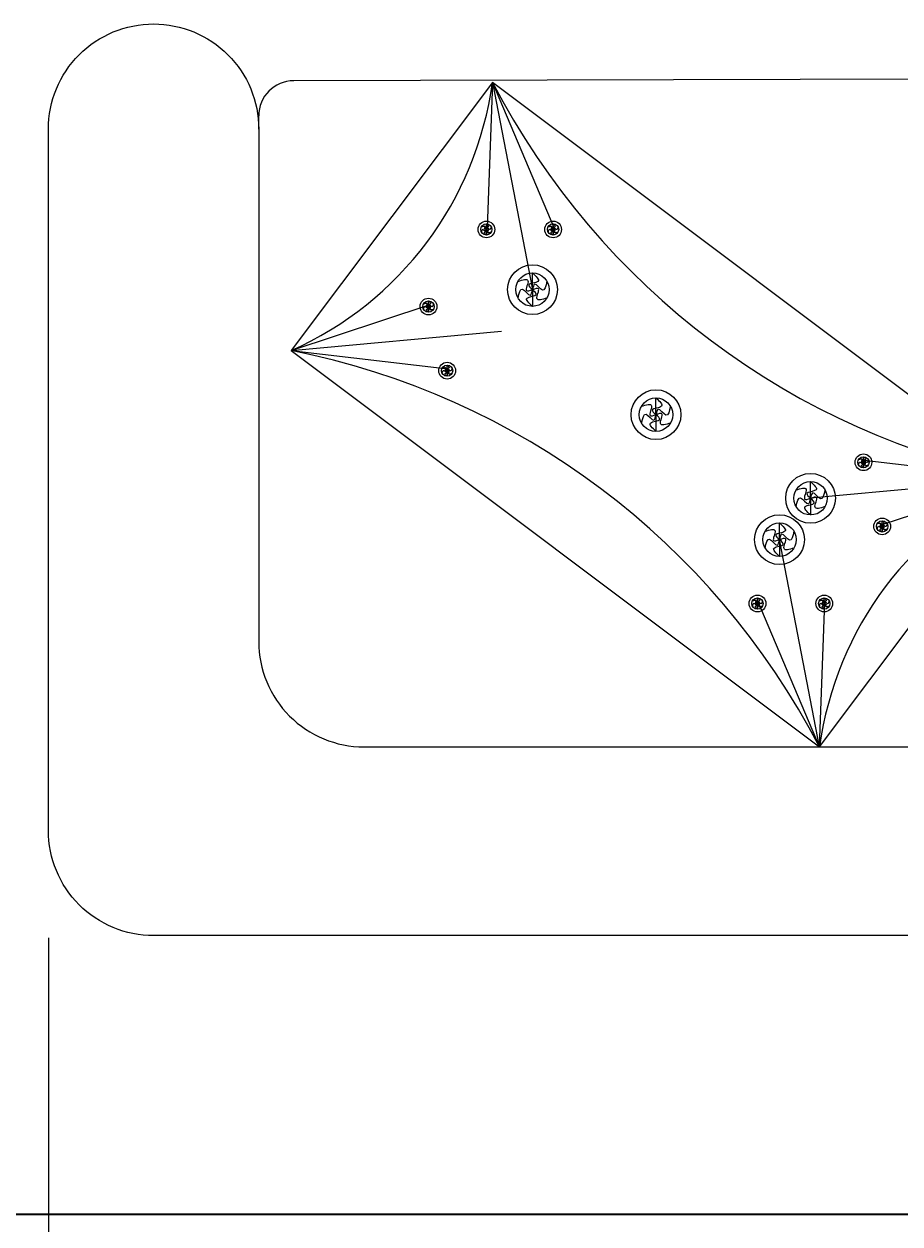
# Model space of a CAD drawing. Units: inches. Extents: x -61 to 1599, y -1316 to 257.
# Tile 163 of 204: x 1123 to 1148, y -939 to -905. Entities that reach past the tile are written whole.
import ezdxf

# ---------------------------------------------------------------- set-up
doc = ezdxf.new("R2010")
doc.units = ezdxf.units.IN
doc.header["$MEASUREMENT"] = 0
for name, color, linetype, lineweight in [('A-ANNO-DIMS', 2, 'Continuous', 18), ('FURNITURE', 83, 'Continuous', 18), ('WALLS', 4, 'Continuous', 35)]:
    doc.layers.add(name, color=color, linetype=linetype, lineweight=lineweight)
doc.layers.add('FUR', color=83, linetype='Continuous')
doc.styles.get("Standard").update_dxf_attribs({"font": 'arial.ttf'})
doc.dimstyles.get("Standard").update_dxf_attribs({"dimtxt": 0.18, "dimasz": 0.18, "dimexe": 0.18, "dimexo": 0.0625, "dimgap": 0.09, "dimtad": 0, "dimtih": 1, "dimtoh": 1, "dimdec": 0, "dimzin": 0, "dimdsep": 46, "dimlunit": 3, "dimtxsty": 'Standard', "dimcen": 0.09, "dimadec": 0, "dimazin": 0, "dimtfac": 1, "dimtdec": 0, "dimtofl": 0, "dimtmove": 0, "dimatfit": 3, "dimfxl": 1, "dimtolj": 1, "dimtzin": 0, "dimarcsym": 0})

# ---------------------------------------------------------------- blocks, each defined once
blk = doc.blocks.new('*U514')
at = {"layer": 'FUR'}
blk.add_open_spline([(0.005, 0.08), (-0.03, 0.048), (-0.098, -0.015), (0.075, -0.018), (0.024, -0.063), (0.005, -0.08)], degree=3, knots=[0, 0, 0, 0, 0.0954578, 0.1898773, 0.2470677, 0.2470677, 0.2470677, 0.2470677], dxfattribs=at)
blk = doc.blocks.new('*U515')
at = {"layer": 'FUR', "transparency": 16777216}
for p, rotation in [((222.173, -79.977), 60), ((222.178, -80.056), 120), ((222.25, -80.092), 180), ((222.312, -79.968), 300), ((222.317, -80.048), 240)]:
    blk.add_blockref('*U514', p, dxfattribs=dict(at, rotation=rotation))
blk.add_blockref('*U514', (222.24, -79.932), dxfattribs=at)
blk = doc.blocks.new('*U516')
at = {"layer": 'FUR'}
blk.add_open_spline([(0.005, 0.08), (-0.03, 0.048), (-0.098, -0.015), (0.075, -0.018), (0.024, -0.063), (0.005, -0.08)], degree=3, knots=[0, 0, 0, 0, 0.0954578, 0.1898773, 0.2470677, 0.2470677, 0.2470677, 0.2470677], dxfattribs=at)
blk = doc.blocks.new('*U517')
at = {"layer": 'FUR', "transparency": 16777216}
for p, rotation in [((222.173, -79.977), 60), ((222.178, -80.056), 120), ((222.25, -80.092), 180), ((222.312, -79.968), 300), ((222.317, -80.048), 240)]:
    blk.add_blockref('*U516', p, dxfattribs=dict(at, rotation=rotation))
blk.add_blockref('*U516', (222.24, -79.932), dxfattribs=at)
blk = doc.blocks.new('*U510')
at = {"layer": 'FUR'}
blk.add_open_spline([(0.005, 0.08), (-0.03, 0.048), (-0.098, -0.015), (0.075, -0.018), (0.024, -0.063), (0.005, -0.08)], degree=3, knots=[0, 0, 0, 0, 0.0954578, 0.1898773, 0.2470677, 0.2470677, 0.2470677, 0.2470677], dxfattribs=at)
blk = doc.blocks.new('*U511')
at = {"layer": 'FUR', "transparency": 16777216}
for p, rotation in [((222.173, -79.977), 60), ((222.178, -80.056), 120), ((222.25, -80.092), 180), ((222.312, -79.968), 300), ((222.317, -80.048), 240)]:
    blk.add_blockref('*U510', p, dxfattribs=dict(at, rotation=rotation))
blk.add_blockref('*U510', (222.24, -79.932), dxfattribs=at)
blk = doc.blocks.new('*U479')
at = {"layer": 'FUR'}
blk.add_open_spline([(0.015, 0.238), (-0.088, 0.143), (-0.292, -0.045), (0.224, -0.053), (0.072, -0.187), (0.015, -0.238)], degree=3, knots=[0, 0, 0, 0, 0.2846533, 0.5662105, 0.736751, 0.736751, 0.736751, 0.736751], dxfattribs=at)
blk = doc.blocks.new('*U480')
at = {"layer": 'FUR', "transparency": 16777216}
blk.add_blockref('*U479', (662.716, -238.357), dxfattribs=at)
for p, rotation in [((662.929, -238.463), 300), ((662.517, -238.489), 60), ((662.531, -238.727), 120), ((662.944, -238.702), 240), ((662.745, -238.833), 180)]:
    blk.add_blockref('*U479', p, dxfattribs=dict(at, rotation=rotation))
blk = doc.blocks.new('*U512')
at = {"layer": 'FUR'}
blk.add_open_spline([(0.005, 0.08), (-0.03, 0.048), (-0.098, -0.015), (0.075, -0.018), (0.024, -0.063), (0.005, -0.08)], degree=3, knots=[0, 0, 0, 0, 0.0954578, 0.1898773, 0.2470677, 0.2470677, 0.2470677, 0.2470677], dxfattribs=at)
blk = doc.blocks.new('*U513')
at = {"layer": 'FUR', "transparency": 16777216}
for p, rotation in [((222.173, -79.977), 60), ((222.178, -80.056), 120), ((222.25, -80.092), 180), ((222.312, -79.968), 300), ((222.317, -80.048), 240)]:
    blk.add_blockref('*U512', p, dxfattribs=dict(at, rotation=rotation))
blk.add_blockref('*U512', (222.24, -79.932), dxfattribs=at)
blk = doc.blocks.new('*U483')
at = {"layer": 'FUR'}
blk.add_open_spline([(0.015, 0.238), (-0.088, 0.143), (-0.292, -0.045), (0.224, -0.053), (0.072, -0.187), (0.015, -0.238)], degree=3, knots=[0, 0, 0, 0, 0.2846533, 0.5662105, 0.736751, 0.736751, 0.736751, 0.736751], dxfattribs=at)
blk = doc.blocks.new('*U484')
at = {"layer": 'FUR', "transparency": 16777216}
blk.add_blockref('*U483', (662.716, -238.357), dxfattribs=at)
for p, rotation in [((662.929, -238.463), 300), ((662.517, -238.489), 60), ((662.531, -238.727), 120), ((662.944, -238.702), 240), ((662.745, -238.833), 180)]:
    blk.add_blockref('*U483', p, dxfattribs=dict(at, rotation=rotation))
blk = doc.blocks.new('*U498')
at = {"layer": 'FUR'}
blk.add_open_spline([(0.005, 0.08), (-0.03, 0.048), (-0.098, -0.015), (0.075, -0.018), (0.024, -0.063), (0.005, -0.08)], degree=3, knots=[0, 0, 0, 0, 0.0954578, 0.1898773, 0.2470677, 0.2470677, 0.2470677, 0.2470677], dxfattribs=at)
blk = doc.blocks.new('*U499')
at = {"layer": 'FUR', "transparency": 16777216}
for p, rotation in [((222.173, -79.977), 60), ((222.178, -80.056), 120), ((222.25, -80.092), 180), ((222.312, -79.968), 300), ((222.317, -80.048), 240)]:
    blk.add_blockref('*U498', p, dxfattribs=dict(at, rotation=rotation))
blk.add_blockref('*U498', (222.24, -79.932), dxfattribs=at)
blk = doc.blocks.new('*U485')
at = {"layer": 'FUR'}
blk.add_open_spline([(0.015, 0.238), (-0.088, 0.143), (-0.292, -0.045), (0.224, -0.053), (0.072, -0.187), (0.015, -0.238)], degree=3, knots=[0, 0, 0, 0, 0.2846533, 0.5662105, 0.736751, 0.736751, 0.736751, 0.736751], dxfattribs=at)
blk = doc.blocks.new('*U497')
at = {"layer": 'FUR', "transparency": 16777216}
blk.add_blockref('*U485', (662.716, -238.357), dxfattribs=at)
for p, rotation in [((662.929, -238.463), 300), ((662.517, -238.489), 60), ((662.531, -238.727), 120), ((662.944, -238.702), 240), ((662.745, -238.833), 180)]:
    blk.add_blockref('*U485', p, dxfattribs=dict(at, rotation=rotation))
blk = doc.blocks.new('*U481')
at = {"layer": 'FUR'}
blk.add_open_spline([(0.015, 0.238), (-0.088, 0.143), (-0.292, -0.045), (0.224, -0.053), (0.072, -0.187), (0.015, -0.238)], degree=3, knots=[0, 0, 0, 0, 0.2846533, 0.5662105, 0.736751, 0.736751, 0.736751, 0.736751], dxfattribs=at)
blk = doc.blocks.new('*U482')
at = {"layer": 'FUR', "transparency": 16777216}
blk.add_blockref('*U481', (662.716, -238.357), dxfattribs=at)
for p, rotation in [((662.929, -238.463), 300), ((662.517, -238.489), 60), ((662.531, -238.727), 120), ((662.944, -238.702), 240), ((662.745, -238.833), 180)]:
    blk.add_blockref('*U481', p, dxfattribs=dict(at, rotation=rotation))
blk = doc.blocks.new('*U477')
at = {"layer": 'FUR'}
blk.add_open_spline([(0.005, 0.08), (-0.03, 0.048), (-0.098, -0.015), (0.075, -0.018), (0.024, -0.063), (0.005, -0.08)], degree=3, knots=[0, 0, 0, 0, 0.0954578, 0.1898773, 0.2470677, 0.2470677, 0.2470677, 0.2470677], dxfattribs=at)
blk = doc.blocks.new('*U478')
at = {"layer": 'FUR', "transparency": 16777216}
for p, rotation in [((222.173, -79.977), 60), ((222.178, -80.056), 120), ((222.25, -80.092), 180), ((222.312, -79.968), 300), ((222.317, -80.048), 240)]:
    blk.add_blockref('*U477', p, dxfattribs=dict(at, rotation=rotation))
blk.add_blockref('*U477', (222.24, -79.932), dxfattribs=at)
blk = doc.blocks.new('*U508')
at = {"layer": 'FUR'}
blk.add_open_spline([(0.005, 0.08), (-0.03, 0.048), (-0.098, -0.015), (0.075, -0.018), (0.024, -0.063), (0.005, -0.08)], degree=3, knots=[0, 0, 0, 0, 0.0954578, 0.1898773, 0.2470677, 0.2470677, 0.2470677, 0.2470677], dxfattribs=at)
blk = doc.blocks.new('*U509')
at = {"layer": 'FUR', "transparency": 16777216}
for p, rotation in [((222.173, -79.977), 60), ((222.178, -80.056), 120), ((222.25, -80.092), 180), ((222.312, -79.968), 300), ((222.317, -80.048), 240)]:
    blk.add_blockref('*U508', p, dxfattribs=dict(at, rotation=rotation))
blk.add_blockref('*U508', (222.24, -79.932), dxfattribs=at)
blk = doc.blocks.new('*U506')
at = {"layer": 'FUR'}
blk.add_open_spline([(0.005, 0.08), (-0.03, 0.048), (-0.098, -0.015), (0.075, -0.018), (0.024, -0.063), (0.005, -0.08)], degree=3, knots=[0, 0, 0, 0, 0.0954578, 0.1898773, 0.2470677, 0.2470677, 0.2470677, 0.2470677], dxfattribs=at)
blk = doc.blocks.new('*U507')
at = {"layer": 'FUR', "transparency": 16777216}
for p, rotation in [((222.173, -79.977), 60), ((222.178, -80.056), 120), ((222.25, -80.092), 180), ((222.312, -79.968), 300), ((222.317, -80.048), 240)]:
    blk.add_blockref('*U506', p, dxfattribs=dict(at, rotation=rotation))
blk.add_blockref('*U506', (222.24, -79.932), dxfattribs=at)
blk = doc.blocks.new('SOFA-THREE-SEAT-ALT-2')
for p, q in [((30, 24.442), (6.996, 24.38)), ((12.664, 24.333), (12.509, 20.191)), ((12.664, 24.333), (13.805, 18.423)), ((12.664, 24.333), (14.414, 20.191)), ((6, 23), (5.999, 23.377)), ((12.49, 20.139), (12.49, 20.299)), ((14.394, 20.139), (14.394, 20.299)), ((12.49, 20.139), (12.49, 19.979)), ((14.394, 20.139), (14.394, 19.979)), ((13.805, 18.423), (13.805, 18.899)), ((13.805, 18.423), (13.805, 17.946)), ((6.926, 16.687), (10.859, 17.993)), ((10.84, 17.94), (10.84, 18.1)), ((10.84, 17.94), (10.84, 17.78)), ((6.926, 16.687), (12.92, 17.243)), ((6.926, 16.687), (11.391, 16.164)), ((11.372, 16.112), (11.372, 16.272)), ((11.372, 16.112), (11.372, 15.952)), ((17.327, 14.857), (17.327, 15.334)), ((17.327, 14.857), (17.327, 14.381)), ((23.243, 13.498), (23.243, 13.658)), ((23.243, 13.498), (23.243, 13.338)), ((27.729, 13.028), (23.263, 13.551)), ((27.729, 13.028), (21.735, 12.472)), ((27.729, 13.028), (23.795, 11.722)), ((21.735, 12.472), (21.735, 12.948)), ((21.735, 12.472), (21.735, 11.995)), ((20.849, 11.292), (20.849, 11.769)), ((23.776, 11.67), (23.776, 11.83)), ((23.776, 11.67), (23.776, 11.51)), ((21.991, 5.382), (20.849, 11.292)), ((20.849, 11.292), (20.849, 10.816)), ((20.221, 9.471), (20.221, 9.631)), ((22.125, 9.471), (22.125, 9.631)), ((20.221, 9.471), (20.221, 9.311)), ((21.991, 5.382), (20.241, 9.523)), ((21.991, 5.382), (22.145, 9.523)), ((22.125, 9.471), (22.125, 9.311))]:
    blk.add_line(p, q)
blk.add_lwpolyline([(78, 8.382), (78, 23, -0.414214), (81, 26), (81, 26, -0.414214), (84, 23), (84, 3, -0.414214), (81, 0), (3, 0, -0.414214), (0, 3), (0, 23, -0.414214), (3, 26), (3, 26, -0.414214), (6, 23), (6, 8.382, 0.414214), (9, 5.382), (75, 5.382, 0.414214)], format="xyb", close=True)
blk.add_lwpolyline([(27.729, 13.028), (12.664, 24.333), (6.926, 16.687), (21.991, 5.382)], close=True)
for centre, radius in [((12.49, 20.139), 0.238), ((12.49, 20.139), 0.16), ((14.394, 20.139), 0.238), ((14.394, 20.139), 0.16), ((13.805, 18.423), 0.71), ((13.805, 18.423), 0.476), ((10.84, 17.94), 0.238), ((10.84, 17.94), 0.16), ((11.372, 16.112), 0.238), ((11.372, 16.112), 0.16), ((17.327, 14.857), 0.71), ((17.327, 14.857), 0.476), ((23.243, 13.498), 0.238), ((23.243, 13.498), 0.16), ((21.735, 12.472), 0.71), ((21.735, 12.472), 0.476), ((20.849, 11.292), 0.71), ((20.849, 11.292), 0.476), ((23.776, 11.67), 0.238), ((23.776, 11.67), 0.16), ((20.221, 9.471), 0.238), ((20.221, 9.471), 0.16), ((22.125, 9.471), 0.238), ((22.125, 9.471), 0.16)]:
    blk.add_circle(centre, radius)
for centre, radius, start, end in [((6.999, 23.38), 1, 90.1542, 180.1542), ((2.937, 25.656), 9.816, 293.9742, 352.253), ((31.951, 34.344), 21.731, 207.4316, 258.7956), ((2.703, -4.63), 21.731, 27.4316, 78.7956), ((31.717, 4.058), 9.816, 113.9742, 172.253)]:
    blk.add_arc(centre, radius, start, end)
at = {"xscale": -1, "rotation": 180}
for name, p in [('*U511', (-209.755, -59.873)), ('*U513', (-207.851, -59.873)), ('*U480', (-648.925, -220.173)), ('*U515', (-211.405, -62.072)), ('*U517', (-210.873, -63.901)), ('*U484', (-645.403, -223.738)), ('*U509', (-199.001, -66.514)), ('*U482', (-640.996, -226.123)), ('*U497', (-641.881, -227.303)), ('*U507', (-198.469, -68.343)), ('*U499', (-202.024, -70.541)), ('*U478', (-200.12, -70.541))]:
    blk.add_blockref(name, p, dxfattribs=at)
blk = doc.blocks.new('*D684')
at = {"layer": 'A-ANNO-DIMS', "color": 0, "lineweight": -2, "transparency": 16777216}
for p, q in [((1123.375, -931.288), (1123.375, -944.005)), ((1207.375, -931.288), (1207.375, -944.005)), ((1123.555, -943.825), (1164.47, -943.825)), ((1207.195, -943.825), (1166.279, -943.825))]:
    blk.add_line(p, q, dxfattribs=at)
at = {"layer": 'A-ANNO-DIMS', "color": 0, "transparency": 16777216}
for points in [[(1123.555, -943.795), (1123.555, -943.855), (1123.375, -943.825)], [(1207.195, -943.795), (1207.195, -943.855), (1207.375, -943.825)]]:
    blk.add_solid(points, dxfattribs=at)
at = {"layer": 'DEFPOINTS', "color": 0, "transparency": 16777216}
for p in [(1123.375, -931.225), (1207.375, -931.225), (1207.375, -943.825)]:
    blk.add_point(p, dxfattribs=at)
at = {"layer": 'A-ANNO-DIMS', "color": 0, "transparency": 16777216, "insert": (1165.375, -943.825), "char_height": 0.18, "attachment_point": 5}
blk.add_mtext('\\A1;SOFA 84 TYP.', dxfattribs=at)

msp = doc.modelspace()

# ---------------------------------------------------------------- linework, layer by layer
at = {"layer": 'WALLS'}
msp.add_line((1097.7028, -939.169), (1212.7028, -939.169), dxfattribs=at)

# ---------------------------------------------------------------- block references
at = {"layer": 'FURNITURE'}
msp.add_blockref('SOFA-THREE-SEAT-ALT-2', (1123.375, -931.225), dxfattribs=at)

# ---------------------------------------------------------------- dimensions: what is measured, and where the dimension line sits
at = {"layer": 'A-ANNO-DIMS'}
dim = msp.add_linear_dim(base=(1207.3746, -943.8253), p1=(1123.3746, -931.2253), p2=(1207.3746, -931.2253), text='SOFA <> TYP.', dimstyle='Standard', override={"dimdec": 0, "dimlfac": 1, "dimrnd": 0, "dimzin": 0, "dimdsep": 46, "dimlunit": 2}, dxfattribs=at)
dim.commit()
dim.dimension.update_dxf_attribs({"geometry": '*D684', "text_midpoint": (1165.3746, -943.8253)})

doc.saveas('drawing.dxf')
